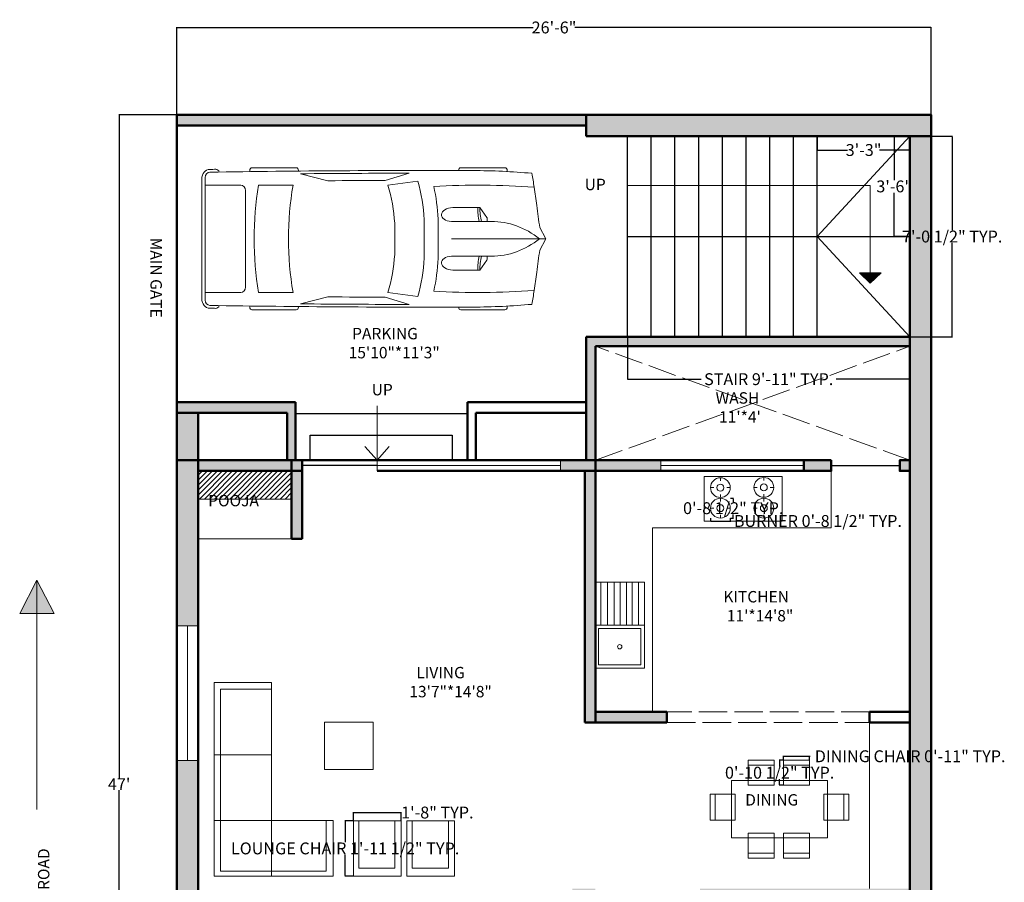
# Model space of a CAD drawing. Units: inches. Extents: x 292 to 1263, y 552 to 1204.
# Tile 2 of 3: x 292 to 707, y 840 to 1204. Entities that reach past the tile are written whole.
import ezdxf

# ---------------------------------------------------------------- set-up
doc = ezdxf.new("R2010")
doc.units = ezdxf.units.IN
doc.header["$MEASUREMENT"] = 0
doc.linetypes.add('ACAD_ISO02W100', pattern=[15, 12, -3])
for name, color, linetype, lineweight in [('A-ANNO-DIMS', 2, 'Continuous', 18), ('A-ANNO-SYMB', 7, 'Continuous', 18), ('A-AREA-IDEN', 30, 'Continuous', 18), ('A-EQPM', 8, 'Continuous', 18), ('A-FLOR-CASE', 92, 'Continuous', 18), ('A-FLOR-CASE-PATT', 252, 'Continuous', 13), ('A-FLOR-FIXT', 9, 'Continuous', 18), ('A-FLOR-OVHD', 8, 'ACAD_ISO02W100', 18), ('A-FLOR-STRS', 7, 'Continuous', 25), ('A-SITE-VEHI', 8, 'Continuous', 18), ('A-WALL-PATT', 22, 'Continuous', 13), ('DOOR', 200, 'Continuous', 25), ('FUR', 92, 'Continuous', 18), ('TEXT', 30, 'Continuous', 18), ('WALL', 22, 'Continuous', 50), ('WIND', 120, 'Continuous', 18)]:
    doc.layers.add(name, color=color, linetype=linetype, lineweight=lineweight)
doc.styles.get("Standard").update_dxf_attribs({"font": 'arial.ttf'})
doc.dimstyles.get("Standard").update_dxf_attribs({"dimtxt": 5, "dimasz": 0.18, "dimexe": 0.18, "dimexo": 0.0625, "dimgap": 0.09, "dimtad": 0, "dimtih": 1, "dimtoh": 1, "dimdec": 0, "dimzin": 0, "dimdsep": 46, "dimlunit": 4, "dimtxsty": 'Standard', "dimcen": 0.09, "dimadec": 0, "dimazin": 0, "dimtfac": 1, "dimtdec": 0, "dimtofl": 0, "dimtmove": 0, "dimatfit": 3, "dimfxl": 1, "dimtolj": 1, "dimtzin": 0, "dimarcsym": 0})

# ---------------------------------------------------------------- blocks, each defined once
blk = doc.blocks.new('*U5')
for p, q in [((46.55, 38.89), (22.35, 38.89)), ((136.7, 38.89), (160.9, 38.89)), ((21.1, 37.41), (21.1, 36.83)), ((47.8, 37.39), (47.8, 37.41)), ((87.99, 31.87), (74.76, 35.92)), ((134.31, 35.6), (119.29, 31.78)), ((135.45, 37.07), (135.45, 37.41)), ((162.15, 37.41), (162.15, 36.77)), ((186.47, -33.5), (186.47, 33.5)), ((188.4, -32.76), (188.4, 32.76)), ((70.03, 31.54), (86.41, 29.35)), ((138.42, 29.35), (157.25, 29.35)), ((186.47, 29.35), (167.01, 29.35)), ((164.52, 26.39), (164.52, -26.39)), ((32.27, 11.63), (36.13, 17.17)), ((36.13, 17.17), (50.94, 17.17)), ((32.12, 9.51), (32.12, 11.15)), ((3.27, 6.13), (0.1, 0.41)), ((29.77, 9.51), (51.68, 9.51)), ((58.92, -10.77), (58.92, 10.77)), ((66.55, -10.53), (66.55, 10.53)), ((82.74, 8.5), (82.74, -8.5)), ((186.47, -10.53), (186.47, 10.53)), ((0, 0), (51.68, 0)), ((0.1, -0.41), (3.27, -6.13)), ((29.77, -9.51), (51.68, -9.51)), ((32.12, -9.51), (32.12, -11.15)), ((32.27, -11.63), (36.13, -17.17)), ((36.13, -17.17), (50.94, -17.17)), ((86.41, -29.35), (70.03, -31.54)), ((87.99, -31.87), (74.76, -35.92)), ((134.31, -35.6), (119.29, -31.78)), ((157.25, -29.35), (138.42, -29.35)), ((167.01, -29.35), (186.47, -29.35)), ((21.1, -37.41), (21.1, -36.83)), ((47.8, -37.39), (47.8, -37.41)), ((135.45, -37.07), (135.45, -37.41)), ((162.15, -37.41), (162.15, -36.77)), ((46.55, -38.89), (22.35, -38.89)), ((136.7, -38.89), (160.9, -38.89))]:
    blk.add_line(p, q)
for centre, major_axis, ratio, start_param, end_param in [((22.35, 37.41), (0, -1.48), 0.842304, 3.141593, 4.712389), ((46.55, 37.41), (0, 1.48), 0.842304, -1.570796, 0), ((136.7, 37.41), (0, -1.48), 0.842304, 3.141593, 4.712389), ((160.9, 37.41), (0, 1.48), 0.842304, -1.570796, 0), ((180.63, 35.84), (0, 2.22), 0.842304, -0.013017, 1.249894), ((64.48, -10556.36), (0, 10595.31), 0.842304, -0.013397, -0.013017), ((183.98, 32.76), (0, -5.25), 0.842304, 1.570796, 3.128196), ((266.03, -27.52), (0, 313.31), 0.842304, 1.367076, 1.39176), ((41.19, -490.86), (0, 528.23), 0.842304, 0.00281, 0.075598), ((64.48, -10555.62), (0, 10593.03), 0.842304, -0.013397, 0.002797), ((64.48, -10555.62), (0, -10591.55), 0.842304, 3.133765, 3.140441), ((183.98, 33.5), (0, -2.96), 0.842304, 1.570796, 3.128196), ((259.18, -27.52), (0, -305.3), 0.842304, 4.528606, 4.561838), ((37.47, -593.96), (0, -623.33), 0.842304, 3.096046, 3.200911), ((134.4, 5.39), (0, -89.78), 0.842304, 4.449482, 4.652344), ((135.29, 5.39), (0, 81.77), 0.842304, 1.245306, 1.50788), ((149.6, 2.8), (0, -79.58), 0.842304, 4.372215, 4.640744), ((95.79, -3666.35), (0, -3698.24), 0.842304, 3.134049, 3.144098), ((17.08, 0), (0, 147.02), 0.842304, 4.511394, 4.913384), ((35.91, 0), (0, 147.02), 0.842304, 4.511394, 4.913384), ((167.01, 26.39), (0, 2.96), 0.842304, 0, 1.570796), ((-204.49, 52.4), (0, -250.96), 0.842304, 1.385369, 1.434372), ((13.04, 17.01), (0, 27.42), 0.842304, 4.435146, 4.718221), ((14.2, 17.01), (0, 27.42), 0.842304, 4.435146, 4.718221), ((50.79, 13.34), (6.34, -0.36), 0.603834, -1.395552, 1.581315), ((32.75, 11.15), (0, 0.74), 0.842304, 0.879714, 1.570796), ((29.77, -46.66), (0, 56.17), 0.842304, 0, 0.590319), ((0.62, 0), (0, -0.74), 0.842304, 4.131459, 5.293319), ((29.77, 46.66), (0, 56.17), 0.842304, 2.551274, 3.141593), ((-204.49, -52.4), (0, 250.96), 0.842304, -1.434372, -1.385369), ((13.04, -17.01), (0, -27.42), 0.842304, 1.564964, 1.848039), ((14.2, -17.01), (0, -27.42), 0.842304, 1.564964, 1.848039), ((134.4, -5.39), (0, -89.78), 0.842304, -1.510751, -1.307889), ((135.29, -5.39), (0, -81.77), 0.842304, -1.50788, -1.245306), ((149.6, -2.8), (0, -79.58), 0.842304, -1.499151, -1.230623), ((32.75, -11.15), (0, -0.74), 0.842304, 4.712389, 5.403472), ((259.18, 27.52), (0, 305.3), 0.842304, 1.721348, 1.754579), ((167.01, -26.39), (0, -2.96), 0.842304, 4.712389, 6.283185), ((266.03, 27.52), (0, 313.31), 0.842304, 1.749832, 1.774517), ((37.47, 593.96), (0, -623.33), 0.842304, -0.059319, 0.045547), ((95.79, 3666.35), (0, -3698.24), 0.842304, -0.002505, 0.007544), ((41.19, 490.86), (0, -528.23), 0.842304, -0.075598, -0.00281), ((22.35, -37.41), (0, 1.48), 0.842304, 1.570796, 3.141593), ((64.48, 10555.62), (0, 10593.03), 0.842304, 3.138796, 3.15499), ((46.55, -37.41), (0, -1.48), 0.842304, 0, 1.570796), ((64.48, 10555.62), (0, -10591.55), 0.842304, 0.001152, 0.007828), ((136.7, -37.41), (0, -1.48), 0.842304, -1.570796, 0), ((160.9, -37.41), (0, 1.48), 0.842304, 3.141593, 4.712389), ((180.63, -35.84), (0, -2.22), 0.842304, -1.249894, 0.013017), ((183.98, -33.5), (0, 2.96), 0.842304, 3.15499, 4.712389), ((183.98, -32.76), (0, -5.25), 0.842304, 0.013397, 1.570796), ((64.48, 10556.36), (0, 10595.31), 0.842304, 3.15461, 3.15499)]:
    blk.add_ellipse(centre, major_axis=major_axis, ratio=ratio, start_param=start_param, end_param=end_param)
at = {"extrusion": (0, 0, -1)}
blk.add_ellipse((50.79, -13.34), major_axis=(6.34, 0.36), ratio=0.603834, start_param=-1.395552, end_param=1.581315, dxfattribs=at)
blk = doc.blocks.new('*D6')
at = {"layer": 'A-ANNO-DIMS', "color": 0, "lineweight": -2, "transparency": 16777216}
for p, q in [((357.97, 1163.71), (357.97, 1200.66)), ((358.15, 1200.48), (508.25, 1200.48)), ((675.79, 1200.48), (525.69, 1200.48)), ((675.97, 1163.71), (675.97, 1200.66))]:
    blk.add_line(p, q, dxfattribs=at)
at = {"layer": 'A-ANNO-DIMS', "color": 0, "lineweight": 100, "transparency": 16777216}
for points in [[(358.15, 1200.51), (358.15, 1200.45), (357.97, 1200.48)], [(675.79, 1200.51), (675.79, 1200.45), (675.97, 1200.48)]]:
    blk.add_solid(points, dxfattribs=at)
at = {"layer": 'Defpoints', "color": 0, "lineweight": 100, "transparency": 16777216}
for p in [(675.97, 1200.48), (357.97, 1163.64), (675.97, 1163.64)]:
    blk.add_point(p, dxfattribs=at)
at = {"layer": 'A-ANNO-DIMS', "color": 0, "transparency": 16777216, "insert": (516.97, 1200.48), "char_height": 5, "attachment_point": 5}
blk.add_mtext('\\A1;26\'-6"', dxfattribs=at)
blk = doc.blocks.new('*D7')
at = {"layer": 'A-ANNO-DIMS', "color": 0, "lineweight": -2, "transparency": 16777216}
for p, q in [((357.91, 1163.64), (333.48, 1163.64)), ((333.66, 1163.46), (333.66, 884.23)), ((333.66, 599.82), (333.66, 879.05)), ((357.91, 599.64), (333.48, 599.64))]:
    blk.add_line(p, q, dxfattribs=at)
at = {"layer": 'A-ANNO-DIMS', "color": 0, "lineweight": 100, "transparency": 16777216}
for points in [[(333.63, 1163.46), (333.69, 1163.46), (333.66, 1163.64)], [(333.63, 599.82), (333.69, 599.82), (333.66, 599.64)]]:
    blk.add_solid(points, dxfattribs=at)
at = {"layer": 'Defpoints', "color": 0, "lineweight": 100, "transparency": 16777216}
for p in [(333.66, 1163.64), (357.97, 1163.64), (357.97, 599.64)]:
    blk.add_point(p, dxfattribs=at)
at = {"layer": 'A-ANNO-DIMS', "color": 0, "transparency": 16777216, "insert": (333.66, 881.64), "char_height": 5, "attachment_point": 5}
blk.add_mtext("\\A1;47'", dxfattribs=at)
blk = doc.blocks.new('*D13')
at = {"layer": 'A-ANNO-DIMS', "color": 0, "lineweight": -2, "transparency": 16777216}
for p, q in [((666.91, 1154.64), (660.2, 1154.64)), ((660.38, 1154.46), (660.38, 1136.16)), ((660.38, 1112.57), (660.38, 1130.87)), ((666.91, 1112.39), (660.2, 1112.39))]:
    blk.add_line(p, q, dxfattribs=at)
at = {"layer": 'A-ANNO-DIMS', "color": 0, "lineweight": 100, "transparency": 16777216}
for points in [[(660.35, 1154.46), (660.41, 1154.46), (660.38, 1154.64)], [(660.35, 1112.57), (660.41, 1112.57), (660.38, 1112.39)]]:
    blk.add_solid(points, dxfattribs=at)
at = {"layer": 'Defpoints', "color": 0, "lineweight": 100, "transparency": 16777216}
for p in [(660.38, 1154.64), (666.97, 1154.64), (666.97, 1112.39)]:
    blk.add_point(p, dxfattribs=at)
at = {"layer": 'A-ANNO-DIMS', "color": 0, "transparency": 16777216, "insert": (660.38, 1133.52), "char_height": 5, "attachment_point": 5}
blk.add_mtext('\\A1;3\'-6"', dxfattribs=at)
blk = doc.blocks.new('*D14')
at = {"layer": 'A-ANNO-DIMS', "color": 0, "lineweight": -2, "transparency": 16777216}
for p, q in [((627.97, 1154.58), (627.97, 1148.67)), ((666.97, 1154.58), (666.97, 1148.67)), ((628.15, 1148.85), (640.73, 1148.85)), ((666.79, 1148.85), (654.2, 1148.85))]:
    blk.add_line(p, q, dxfattribs=at)
at = {"layer": 'A-ANNO-DIMS', "color": 0, "lineweight": 100, "transparency": 16777216}
for points in [[(628.15, 1148.88), (628.15, 1148.82), (627.97, 1148.85)], [(666.79, 1148.88), (666.79, 1148.82), (666.97, 1148.85)]]:
    blk.add_solid(points, dxfattribs=at)
at = {"layer": 'Defpoints', "color": 0, "lineweight": 100, "transparency": 16777216}
for p in [(627.97, 1154.64), (666.97, 1154.64), (666.97, 1148.85)]:
    blk.add_point(p, dxfattribs=at)
at = {"layer": 'A-ANNO-DIMS', "color": 0, "transparency": 16777216, "insert": (647.47, 1148.85), "char_height": 5, "attachment_point": 5}
blk.add_mtext('\\A1;3\'-3"', dxfattribs=at)
blk = doc.blocks.new('SOFA-SECTIONAL')
for p, q in [((2.73, 2.04), (2.73, 78.73)), ((2.73, 78.73), (24.15, 78.73)), ((24.15, 51.12), (0, 51.12)), ((47.26, 23.35), (47.26, 2.04)), ((47.26, 2.04), (2.73, 2.04))]:
    blk.add_line(p, q)
for points in [[(0, 0), (24.15, 0), (24.15, 81.48), (0, 81.48)], [(0, 0), (50.13, 0), (50.13, 23.35), (0, 23.35)]]:
    blk.add_lwpolyline(points, close=True)
blk = doc.blocks.new('CHAIR-LOUNGE')
for p, q in [((2.25, 23.26), (2.25, 3.36)), ((17.47, 3.36), (17.47, 23.26)), ((2.25, 3.36), (17.47, 3.36))]:
    blk.add_line(p, q)
blk.add_lwpolyline([(0, 0), (20.12, 0), (20.12, 23.26), (0, 23.26)], close=True)
blk = doc.blocks.new('CHAIR-DINING')
blk.add_line((0, 8.43), (11, 8.43))
blk.add_lwpolyline([(0, 0), (11, 0), (11, 10.56), (0, 10.56)], close=True)
blk = doc.blocks.new('COOKTOP-BURNER')
for p, q in [((4.16, 8.32), (4.16, 7.02)), ((0, 4.16), (0.93, 4.16)), ((0, 4.16), (1.41, 4.16)), ((6.9, 4.16), (8.32, 4.16)), ((4.16, 1.29), (4.16, 0))]:
    blk.add_line(p, q)
for radius in [4.16, 1.47]:
    blk.add_circle((4.16, 4.16), radius)
blk = doc.blocks.new('STAIR-RETURN')
for p, q in [((0, 0), (0, 84.5)), ((10, 0), (10, 84.5)), ((20, 0), (20, 84.5)), ((30, 0), (30, 84.5)), ((40, 0), (40, 84.5)), ((50, 0), (50, 84.5)), ((60, 0), (60, 84.5)), ((70, 0), (70, 84.5)), ((80, 0), (80, 84.5)), ((80, 42.25), (119, 84.5)), ((0, 42.25), (119, 42.25)), ((80, 42.25), (119, 0)), ((80, 0), (80, 39))]:
    blk.add_line(p, q)
blk = doc.blocks.new('STAIR-TRAVEL-ARROW')
h = blk.add_hatch()
h.set_pattern_fill('ANSI31', color=256)
h.set_pattern_definition([(45, (-547.968, -1092.695), (-0.088388348, 0.088388348), [])])
h.paths.add_polyline_path([(102.33, 4.46), (97.71, 4.46), (102.33, 0)])
h.paths.add_polyline_path([(106.95, 4.46), (102.33, 4.46), (102.33, 0)])
for p, q in [((0, 41.14), (102.33, 41.14)), ((102.33, 41.14), (102.33, 0)), ((102.33, 0), (97.71, 4.46)), ((97.71, 4.46), (106.95, 4.46)), ((102.33, 0), (106.95, 4.46))]:
    blk.add_line(p, q)
blk = doc.blocks.new('ROAD-DIRECTION')
h = blk.add_hatch(color=256)
h.dxf.hatch_style = 1
h.paths.add_polyline_path([(7.26, 265.02), (0, 250.97), (7.26, 250.97)])
h.paths.add_polyline_path([(7.26, 265.02), (7.26, 250.97), (14.53, 250.97)])
h.paths.add_polyline_path([(14.53, 14.04), (7.26, 14.04), (7.26, 0)])
h.paths.add_polyline_path([(7.26, 14.04), (0, 14.04), (7.26, 0)])
for p, q in [((7.26, 265.02), (0, 250.97)), ((7.26, 168.49), (7.26, 265.02)), ((7.26, 265.02), (14.53, 250.97)), ((0, 250.97), (14.53, 250.97)), ((7.26, 96.52), (7.26, 0)), ((7.26, 0), (0, 14.04)), ((0, 14.04), (14.53, 14.04)), ((7.26, 0), (14.53, 14.04))]:
    blk.add_line(p, q)
blk = doc.blocks.new('WASH-VOID')
for p, q in [((0, 0), (132.5, 48)), ((132.5, 0), (0, 48))]:
    blk.add_line(p, q)
blk = doc.blocks.new('WIN-SIDE')
blk.add_line((4.5, 0), (4.5, 56.83))
blk.add_lwpolyline([(9, 56.83), (0, 56.83), (0, 0), (9, 0)], close=True)
blk = doc.blocks.new('*D29')
at = {"layer": 'A-ANNO-DIMS', "color": 0, "lineweight": -2, "transparency": 16777216}
for p, q in [((613.73, 891.82), (613.73, 893.58)), ((613.91, 893.4), (624.55, 893.4)), ((624.73, 891.82), (624.73, 893.58)), ((624.73, 893.4), (624.91, 893.4))]:
    blk.add_line(p, q, dxfattribs=at)
at = {"layer": 'A-ANNO-DIMS', "color": 0, "lineweight": 100, "transparency": 16777216}
for points in [[(613.91, 893.43), (613.91, 893.37), (613.73, 893.4)], [(624.55, 893.43), (624.55, 893.37), (624.73, 893.4)]]:
    blk.add_solid(points, dxfattribs=at)
at = {"layer": 'Defpoints', "color": 0, "lineweight": 100, "transparency": 16777216}
for p in [(624.73, 893.4), (613.73, 891.75), (624.73, 891.75)]:
    blk.add_point(p, dxfattribs=at)
at = {"layer": 'A-ANNO-DIMS', "color": 0, "transparency": 16777216, "insert": (667.09, 893.4), "char_height": 5, "attachment_point": 5}
blk.add_mtext('\\A1;DINING CHAIR 0\'-11" TYP.', dxfattribs=at)
blk = doc.blocks.new('*D30')
at = {"layer": 'A-ANNO-DIMS', "color": 0, "lineweight": -2, "transparency": 16777216}
for p, q in [((613.67, 891.75), (611.9, 891.75)), ((612.08, 891.57), (612.08, 889.15)), ((613.67, 881.19), (611.9, 881.19)), ((612.08, 881.37), (612.08, 883.8))]:
    blk.add_line(p, q, dxfattribs=at)
at = {"layer": 'A-ANNO-DIMS', "color": 0, "lineweight": 100, "transparency": 16777216}
for points in [[(612.05, 891.57), (612.11, 891.57), (612.08, 891.75)], [(612.05, 881.37), (612.11, 881.37), (612.08, 881.19)]]:
    blk.add_solid(points, dxfattribs=at)
at = {"layer": 'Defpoints', "color": 0, "lineweight": 100, "transparency": 16777216}
for p in [(612.08, 891.75), (613.73, 891.75), (613.73, 881.19)]:
    blk.add_point(p, dxfattribs=at)
at = {"layer": 'A-ANNO-DIMS', "color": 0, "transparency": 16777216, "insert": (612.08, 886.47), "char_height": 5, "attachment_point": 5}
blk.add_mtext('\\A1;0\'-10 1/2" TYP.', dxfattribs=at)
blk = doc.blocks.new('*D31')
at = {"layer": 'A-ANNO-DIMS', "color": 0, "lineweight": -2, "transparency": 16777216}
for p, q in [((582.96, 993.71), (582.96, 992.35)), ((583.14, 992.53), (591.09, 992.53)), ((591.27, 993.71), (591.27, 992.35)), ((591.27, 992.53), (591.45, 992.53))]:
    blk.add_line(p, q, dxfattribs=at)
at = {"layer": 'A-ANNO-DIMS', "color": 0, "lineweight": 100, "transparency": 16777216}
for points in [[(583.14, 992.56), (583.14, 992.5), (582.96, 992.53)], [(591.09, 992.56), (591.09, 992.5), (591.27, 992.53)]]:
    blk.add_solid(points, dxfattribs=at)
at = {"layer": 'Defpoints', "color": 0, "lineweight": 100, "transparency": 16777216}
for p in [(582.96, 993.78), (591.27, 993.78), (591.27, 992.53)]:
    blk.add_point(p, dxfattribs=at)
at = {"layer": 'A-ANNO-DIMS', "color": 0, "transparency": 16777216, "insert": (628.21, 992.53), "char_height": 5, "attachment_point": 5}
blk.add_mtext('\\A1;BURNER 0\'-8 1/2" TYP.', dxfattribs=at)
blk = doc.blocks.new('*D32')
at = {"layer": 'A-ANNO-DIMS', "color": 0, "lineweight": -2, "transparency": 16777216}
for p, q in [((591.33, 1002.09), (592.7, 1002.09)), ((592.52, 1001.91), (592.52, 1000.61)), ((591.33, 993.78), (592.7, 993.78)), ((592.52, 993.96), (592.52, 995.26))]:
    blk.add_line(p, q, dxfattribs=at)
at = {"layer": 'A-ANNO-DIMS', "color": 0, "lineweight": 100, "transparency": 16777216}
for points in [[(592.49, 1001.91), (592.55, 1001.91), (592.52, 1002.09)], [(592.49, 993.96), (592.55, 993.96), (592.52, 993.78)]]:
    blk.add_solid(points, dxfattribs=at)
at = {"layer": 'Defpoints', "color": 0, "lineweight": 100, "transparency": 16777216}
for p in [(591.27, 1002.09), (592.52, 1002.09), (591.27, 993.78)]:
    blk.add_point(p, dxfattribs=at)
at = {"layer": 'A-ANNO-DIMS', "color": 0, "transparency": 16777216, "insert": (592.52, 997.94), "char_height": 5, "attachment_point": 5}
blk.add_mtext('\\A1;0\'-8 1/2" TYP.', dxfattribs=at)
blk = doc.blocks.new('*D37')
at = {"layer": 'A-ANNO-DIMS', "color": 0, "lineweight": -2, "transparency": 16777216}
for p, q in [((432.33, 866.2), (428.73, 866.2)), ((428.91, 866.02), (428.91, 857.25)), ((428.91, 843.12), (428.91, 851.9)), ((432.33, 842.94), (428.73, 842.94))]:
    blk.add_line(p, q, dxfattribs=at)
at = {"layer": 'A-ANNO-DIMS', "color": 0, "lineweight": 100, "transparency": 16777216}
for points in [[(428.88, 866.02), (428.94, 866.02), (428.91, 866.2)], [(428.88, 843.12), (428.94, 843.12), (428.91, 842.94)]]:
    blk.add_solid(points, dxfattribs=at)
at = {"layer": 'Defpoints', "color": 0, "lineweight": 100, "transparency": 16777216}
for p in [(428.91, 866.2), (432.4, 866.2), (432.4, 842.94)]:
    blk.add_point(p, dxfattribs=at)
at = {"layer": 'A-ANNO-DIMS', "color": 0, "transparency": 16777216, "insert": (428.91, 854.57), "char_height": 5, "attachment_point": 5}
blk.add_mtext('\\A1;LOUNGE CHAIR 1\'-11 1/2" TYP.', dxfattribs=at)
blk = doc.blocks.new('*D38')
at = {"layer": 'A-ANNO-DIMS', "color": 0, "lineweight": -2, "transparency": 16777216}
for p, q in [((432.4, 866.27), (432.4, 869.87)), ((432.58, 869.69), (452.33, 869.69)), ((452.51, 866.27), (452.51, 869.87)), ((452.51, 869.69), (452.69, 869.69))]:
    blk.add_line(p, q, dxfattribs=at)
at = {"layer": 'A-ANNO-DIMS', "color": 0, "lineweight": 100, "transparency": 16777216}
for points in [[(432.58, 869.72), (432.58, 869.66), (432.4, 869.69)], [(452.33, 869.72), (452.33, 869.66), (452.51, 869.69)]]:
    blk.add_solid(points, dxfattribs=at)
at = {"layer": 'Defpoints', "color": 0, "lineweight": 100, "transparency": 16777216}
for p in [(452.51, 869.69), (432.4, 866.2), (452.51, 866.2)]:
    blk.add_point(p, dxfattribs=at)
at = {"layer": 'A-ANNO-DIMS', "color": 0, "transparency": 16777216, "insert": (467.79, 869.69), "char_height": 5, "attachment_point": 5}
blk.add_mtext('\\A1;1\'-8" TYP.', dxfattribs=at)
blk = doc.blocks.new('*D39')
at = {"layer": 'A-ANNO-DIMS', "color": 0, "lineweight": -2, "transparency": 16777216}
for p, q in [((547.97, 1070.08), (547.97, 1052.11)), ((666.97, 1070.08), (666.97, 1052.11)), ((548.15, 1052.29), (578.95, 1052.29)), ((666.79, 1052.29), (635.98, 1052.29))]:
    blk.add_line(p, q, dxfattribs=at)
at = {"layer": 'A-ANNO-DIMS', "color": 0, "lineweight": 100, "transparency": 16777216}
for points in [[(548.15, 1052.32), (548.15, 1052.26), (547.97, 1052.29)], [(666.79, 1052.32), (666.79, 1052.26), (666.97, 1052.29)]]:
    blk.add_solid(points, dxfattribs=at)
at = {"layer": 'Defpoints', "color": 0, "lineweight": 100, "transparency": 16777216}
for p in [(547.97, 1070.14), (666.97, 1070.14), (666.97, 1052.29)]:
    blk.add_point(p, dxfattribs=at)
at = {"layer": 'A-ANNO-DIMS', "color": 0, "transparency": 16777216, "insert": (607.47, 1052.29), "char_height": 5, "attachment_point": 5}
blk.add_mtext('\\A1;STAIR 9\'-11" TYP.', dxfattribs=at)
blk = doc.blocks.new('*D40')
at = {"layer": 'A-ANNO-DIMS', "color": 0, "lineweight": -2, "transparency": 16777216}
for p, q in [((667.03, 1154.64), (685, 1154.64)), ((684.82, 1154.46), (684.82, 1115.07)), ((684.82, 1070.32), (684.82, 1109.72)), ((667.03, 1070.14), (685, 1070.14))]:
    blk.add_line(p, q, dxfattribs=at)
at = {"layer": 'A-ANNO-DIMS', "color": 0, "lineweight": 100, "transparency": 16777216}
for points in [[(684.79, 1154.46), (684.85, 1154.46), (684.82, 1154.64)], [(684.79, 1070.32), (684.85, 1070.32), (684.82, 1070.14)]]:
    blk.add_solid(points, dxfattribs=at)
at = {"layer": 'Defpoints', "color": 0, "lineweight": 100, "transparency": 16777216}
for p in [(666.97, 1154.64), (684.82, 1154.64), (666.97, 1070.14)]:
    blk.add_point(p, dxfattribs=at)
at = {"layer": 'A-ANNO-DIMS', "color": 0, "transparency": 16777216, "insert": (684.82, 1112.39), "char_height": 5, "attachment_point": 5}
blk.add_mtext('\\A1;7\'-0 1/2" TYP.', dxfattribs=at)

msp = doc.modelspace()

# ---------------------------------------------------------------- hatches: boundary and pattern name
at = {"layer": 'A-FLOR-CASE-PATT'}
h = msp.add_hatch(dxfattribs=at)
h.set_pattern_fill('ANSI31', color=256, scale=12)
h.paths.add_polyline_path([(406.28, 1013.64), (366.97, 1013.64), (366.97, 1001.8), (406.28, 1001.8)])
at = {"layer": 'A-WALL-PATT'}
h = msp.add_hatch(color=256, dxfattribs=at)
h.dxf.hatch_style = 1
h.paths.add_polyline_path([(530.47, 1163.64), (357.97, 1163.64), (357.97, 1159.14), (530.47, 1159.14)])
h.paths.add_polyline_path([(407.97, 1042.64), (357.97, 1042.64), (357.97, 1038.14), (404.42, 1038.14), (404.42, 1018.14), (407.97, 1018.14)])
h = msp.add_hatch(color=256, dxfattribs=at)
h.dxf.hatch_style = 1
h.paths.add_polyline_path([(675.97, 1163.64), (530.47, 1163.64), (530.47, 1154.64), (675.97, 1154.64)])
h = msp.add_hatch(color=256, dxfattribs=at)
h.dxf.hatch_style = 1
h.paths.add_polyline_path([(675.97, 1154.64), (666.97, 1154.64), (666.97, 599.64), (675.97, 599.64)])
h.paths.add_polyline_path([(666.97, 608.64), (644.63, 608.64), (644.63, 599.64), (666.97, 599.64)])
h.paths.add_polyline_path([(469.97, 713.14), (406.46, 713.14), (406.46, 708.64), (469.97, 708.64)])
h = msp.add_hatch(color=256, dxfattribs=at)
h.dxf.hatch_style = 1
h.paths.add_polyline_path([(534.47, 1013.64), (529.97, 1013.64), (529.97, 907.64), (534.47, 907.64)])
h.paths.add_polyline_path([(666.97, 1070.14), (627.97, 1070.14), (530.47, 1070.14), (530.47, 1018.14), (534.47, 1018.14), (534.47, 1066.14), (666.97, 1066.14)])
h.paths.add_polyline_path([(633.82, 1018.14), (622.22, 1018.14), (622.22, 1013.64), (633.82, 1013.64)])
h.paths.add_polyline_path([(562.03, 1018.14), (534.97, 1018.14), (534.47, 1018.14), (534.47, 1013.64), (562.03, 1013.64)])
h.paths.add_polyline_path([(666.97, 1018.14), (662.7, 1018.14), (662.7, 1013.64), (666.97, 1013.64)])
h.paths.add_polyline_path([(534.47, 1018.14), (519.71, 1018.14), (519.71, 1013.64), (529.97, 1013.64), (534.47, 1013.64)])
h = msp.add_hatch(color=256, dxfattribs=at)
h.dxf.hatch_style = 1
h.paths.add_polyline_path([(366.97, 1038.14), (357.97, 1038.14), (357.97, 1018.14), (366.97, 1018.14)])
h.paths.add_polyline_path([(366.97, 1013.64), (366.97, 1018.14), (357.97, 1018.14), (357.97, 948.4), (366.97, 948.4)])
h.paths.add_polyline_path([(366.97, 891.57), (357.97, 891.57), (357.97, 803.1), (366.97, 803.1), (366.97, 833.14)])
h.paths.add_polyline_path([(366.97, 746.27), (357.97, 746.27), (357.97, 702.82), (366.97, 702.82), (366.97, 708.64)])
h.paths.add_polyline_path([(381.13, 608.64), (367.97, 608.64), (366.97, 608.64), (366.97, 618.29), (357.97, 618.29), (357.97, 599.64), (381.13, 599.64)])
h.paths.add_polyline_path([(492.73, 608.64), (474.47, 608.64), (469.6, 608.64), (469.6, 599.64), (492.73, 599.64)])
h.paths.add_polyline_path([(560.01, 608.64), (516.97, 608.64), (516.97, 599.64), (560.01, 599.64)])
h.paths.add_polyline_path([(474.47, 708.64), (474.47, 713.14), (469.97, 713.14), (469.97, 608.64), (474.47, 608.64)])
h.paths.add_polyline_path([(534.97, 764.64), (534.92, 775.88), (534.43, 837.64), (524.76, 837.64), (524.76, 833.14), (529.97, 833.14), (530.47, 769.14), (530.47, 608.64), (534.97, 608.64)])
h.paths.add_polyline_path([(582.97, 769.14), (582.97, 775.01), (578.47, 775.01), (578.47, 769.14), (578.47, 739.47), (582.97, 739.47), (582.97, 764.64)])
h.paths.add_polyline_path([(666.97, 769.14), (642.97, 769.14), (582.97, 769.14), (582.97, 764.64), (666.97, 764.64)])
h.paths.add_polyline_path([(666.97, 837.64), (578.47, 837.64), (578.47, 816.16), (578.47, 815.01), (582.97, 815.01), (582.97, 816.16), (582.97, 833.14), (666.97, 833.14)])
h.paths.add_polyline_path([(564.59, 912.14), (534.47, 912.14), (534.47, 907.64), (564.59, 907.64)])
h = msp.add_hatch(color=256, dxfattribs=at)
h.dxf.hatch_style = 1
h.paths.add_polyline_path([(410.78, 1013.64), (406.28, 1013.64), (406.28, 984.99), (410.78, 984.99)])
h.paths.add_polyline_path([(410.78, 1018.14), (406.28, 1018.14), (406.28, 1013.64), (410.78, 1013.64)])
h.paths.add_polyline_path([(406.28, 1018.14), (366.97, 1018.14), (366.97, 1013.64), (406.28, 1013.64)])

# ---------------------------------------------------------------- linework, layer by layer
at = {"layer": 'A-ANNO-SYMB'}
for p, q in [((442.36, 1037.79), (442.36, 1041.1)), ((442.36, 1018.14), (442.36, 1037.79)), ((442.36, 1018.14), (437.25, 1023.93)), ((442.36, 1018.14), (447.46, 1023.93))]:
    msp.add_line(p, q, dxfattribs=at)
at = {"layer": 'A-EQPM'}
msp.add_lwpolyline([(580.24, 1011.26), (613.12, 1011.26), (613.12, 992.46), (580.24, 992.46)], close=True, dxfattribs=at)
at = {"layer": 'A-FLOR-CASE'}
for p, q in [((633.82, 1013.64), (633.82, 989.64)), ((366.97, 1001.8), (406.28, 1001.8)), ((633.82, 989.64), (558.47, 989.64)), ((558.47, 912.14), (558.47, 989.64)), ((406.28, 984.99), (366.97, 984.99)), ((534.47, 912.14), (558.47, 912.14)), ((650.02, 907.64), (650.02, 837.64))]:
    msp.add_line(p, q, dxfattribs=at)
at = {"layer": 'A-FLOR-FIXT'}
for p, q in [((536.76, 948.66), (536.76, 966.8)), ((539.45, 948.66), (539.45, 966.8)), ((542.32, 948.66), (542.32, 966.8)), ((544.92, 948.66), (544.92, 966.8)), ((547.52, 948.67), (547.52, 966.81)), ((549.94, 948.67), (549.94, 966.81)), ((552.54, 948.66), (552.54, 966.8)), ((555.11, 948.66), (534.47, 948.66))]:
    msp.add_line(p, q, dxfattribs=at)
for points in [[(555.11, 966.8), (534.47, 966.8), (534.47, 930.52), (555.11, 930.52)], [(535.78, 931.94), (553.61, 931.94), (553.61, 947.17), (535.78, 947.17)]]:
    msp.add_lwpolyline(points, close=True, dxfattribs=at)
msp.add_circle((544.69, 939.56), 0.924, dxfattribs=at)
at = {"layer": 'A-FLOR-OVHD'}
msp.add_lwpolyline([(564.59, 907.64), (650.02, 907.64), (650.02, 912.14), (564.59, 912.14)], close=True, dxfattribs=at)
at = {"layer": 'A-FLOR-STRS'}
for p, q in [((666.97, 1070.14), (627.97, 1070.14)), ((666.97, 1070.14), (627.97, 1070.14)), ((407.97, 1037.79), (480.47, 1037.79)), ((414.2, 1018.14), (414.2, 1028.7)), ((414.2, 1028.7), (473.97, 1028.7)), ((473.97, 1028.7), (473.97, 1018.14))]:
    msp.add_line(p, q, dxfattribs=at)
at = {"layer": 'DOOR'}
for p, q in [((442.36, 1015.89), (410.78, 1015.89)), ((633.82, 1015.89), (662.7, 1015.89))]:
    msp.add_line(p, q, dxfattribs=at)
at = {"layer": 'FUR'}
for points in [[(420.2, 907.83), (440.72, 907.83), (440.72, 887.85), (420.2, 887.85)], [(591.83, 883.13), (632.25, 883.13), (632.25, 859.07), (591.83, 859.07)]]:
    msp.add_lwpolyline(points, close=True, dxfattribs=at)
at = {"layer": 'WALL'}
for p, q in [((357.97, 1163.64), (675.97, 1163.64)), ((357.97, 1163.64), (357.97, 1159.14)), ((357.97, 1018.14), (357.97, 1163.64)), ((530.47, 1154.64), (530.47, 1163.64)), ((675.97, 599.64), (675.97, 1163.64)), ((530.47, 1159.14), (357.97, 1159.14)), ((530.47, 1154.64), (666.97, 1154.64)), ((666.97, 608.64), (666.97, 1154.64)), ((530.47, 1018.14), (530.47, 1070.14)), ((530.47, 1070.14), (666.97, 1070.14)), ((534.47, 1018.14), (534.47, 1066.14)), ((534.47, 1066.14), (666.97, 1066.14)), ((357.97, 1042.64), (407.97, 1042.64)), ((407.97, 1042.64), (407.97, 1018.14)), ((530.47, 1042.64), (480.47, 1042.64)), ((480.47, 1042.64), (480.47, 1018.14)), ((357.97, 1018.14), (357.97, 1038.14)), ((357.97, 1038.14), (404.42, 1038.14)), ((366.97, 1018.14), (366.97, 1038.14)), ((404.42, 1018.14), (404.42, 1038.14)), ((530.47, 1038.14), (484.01, 1038.14)), ((484.01, 1018.14), (484.01, 1038.14)), ((366.97, 1018.14), (357.97, 1018.14)), ((357.97, 1018.14), (357.97, 599.64)), ((366.97, 1018.14), (366.97, 608.64)), ((366.97, 1018.14), (534.47, 1018.14)), ((406.28, 1018.14), (406.28, 984.99)), ((410.78, 1018.14), (410.78, 984.99)), ((529.97, 1018.14), (633.82, 1018.14)), ((534.47, 1018.14), (534.47, 907.64)), ((633.82, 1018.14), (534.97, 1018.14)), ((666.97, 1018.14), (662.7, 1018.14)), ((662.7, 1018.14), (666.97, 1018.14)), ((366.97, 837.64), (366.97, 1013.64)), ((366.97, 1013.64), (410.78, 1013.64)), ((442.36, 1013.64), (529.97, 1013.64)), ((529.97, 1013.64), (529.97, 907.64)), ((529.97, 1013.64), (633.82, 1013.64)), ((534.47, 1013.64), (534.47, 907.64)), ((662.7, 1013.64), (666.97, 1013.64)), ((406.28, 984.99), (410.78, 984.99)), ((564.59, 912.14), (534.47, 912.14)), ((666.97, 912.14), (650.02, 912.14)), ((534.47, 907.64), (529.97, 907.64)), ((564.59, 907.64), (534.47, 907.64)), ((666.97, 907.64), (650.02, 907.64))]:
    msp.add_line(p, q, dxfattribs=at)
for points in [[(530.47, 1154.64), (675.97, 1154.64), (675.97, 1163.64), (530.47, 1163.64)], [(666.97, 1154.64), (675.97, 1154.64), (675.97, 599.64), (666.97, 599.64)], [(633.82, 1018.14), (622.22, 1018.14), (622.22, 1013.64), (633.82, 1013.64)], [(666.97, 1018.14), (662.7, 1018.14), (662.7, 1013.64), (666.97, 1013.64)]]:
    msp.add_lwpolyline(points, close=True, dxfattribs=at)
for points in [[(564.59, 912.14), (564.59, 907.64)], [(650.02, 907.64), (650.02, 912.14)]]:
    msp.add_lwpolyline(points, dxfattribs=at)
at = {"layer": 'WIND'}
for p, q in [((442.36, 1015.89), (519.71, 1015.89)), ((562.03, 1015.89), (622.22, 1015.89))]:
    msp.add_line(p, q, dxfattribs=at)
for points in [[(519.71, 1013.64), (442.36, 1013.64), (442.36, 1018.14), (519.71, 1018.14)], [(622.22, 1013.64), (562.03, 1013.64), (562.03, 1018.14), (622.22, 1018.14)]]:
    msp.add_lwpolyline(points, close=True, dxfattribs=at)
msp.add_lwpolyline([(473.94, 1013.64), (519.71, 1013.64), (519.71, 1018.14), (473.94, 1018.14)], dxfattribs=at)

# ---------------------------------------------------------------- block references
at = {"layer": 'A-ANNO-SYMB'}
for name, p in [('STAIR-TRAVEL-ARROW', (547.97, 1092.69)), ('ROAD-DIRECTION', (291.73, 702.52))]:
    msp.add_blockref(name, p, dxfattribs=at)
at = {"layer": 'A-EQPM'}
for p in [(582.96, 1002.42), (601.26, 1002.54), (582.96, 993.78), (601.26, 993.78)]:
    msp.add_blockref('COOKTOP-BURNER', p, dxfattribs=at)
at = {"layer": 'A-FLOR-OVHD'}
msp.add_blockref('WASH-VOID', (534.47, 1018.14), dxfattribs=at)
at = {"layer": 'A-FLOR-STRS'}
msp.add_blockref('STAIR-RETURN', (547.97, 1070.14), dxfattribs=at)
at = {"layer": 'A-SITE-VEHI', "xscale": -0.7697678212056502, "yscale": 0.7697678212056502, "zscale": 0.7697678212056502}
msp.add_blockref('*U5', (513.5, 1111.43), dxfattribs=at)
at = {"layer": 'FUR'}
for name, p in [('SOFA-SECTIONAL', (373.7, 842.94)), ('CHAIR-DINING', (598.8, 881.19)), ('CHAIR-DINING', (613.73, 881.19)), ('CHAIR-LOUNGE', (432.4, 842.94)), ('CHAIR-LOUNGE', (454.97, 842.94))]:
    msp.add_blockref(name, p, dxfattribs=at)
at = {"layer": 'FUR', "rotation": 90}
msp.add_blockref('CHAIR-DINING', (593.33, 866.49), dxfattribs=at)
at = {"layer": 'FUR', "extrusion": (0, 0, -1), "zscale": -1}
for p, rotation in [((-630.75, 866.49), 90.0000000000006), ((-598.8, 861.01), 180), ((-613.73, 861.01), 180)]:
    msp.add_blockref('CHAIR-DINING', p, dxfattribs=dict(at, rotation=rotation))
at = {"layer": 'WIND'}
msp.add_blockref('WIN-SIDE', (357.97, 891.57), dxfattribs=at)

# ---------------------------------------------------------------- texts
at = {"layer": 'A-AREA-IDEN', "attachment_point": 1}
for s, insert, char_height in [(' PARKING \\P15\'10"*11\'3"', (430.41, 1073.89), 4.8055), ("WASH\\P 11'*4'", (585.08, 1046.78), 4.805), ('POOJA', (371.2, 1003.52), 4.805), ('KITCHEN\\P 11\'*14\'8"', (588.37, 963.03), 4.805), ('  LIVING\\P13\'7"*14\'8"', (455.99, 931.05), 4.8055), ('DINING', (597.58, 877.43), 4.805)]:
    msp.add_mtext_dynamic_manual_height_columns(s, width=2330.1292, gutter_width=24.03, heights=[0], dxfattribs=dict(at, insert=insert, char_height=char_height))
at = {"layer": 'TEXT', "char_height": 4.805, "attachment_point": 1}
for insert in [(529.9, 1136.74), (440.12, 1050.28)]:
    msp.add_mtext_dynamic_manual_height_columns('UP', width=2330.1292, gutter_width=24.03, heights=[0], dxfattribs=dict(at, insert=insert))
for s, insert, rotation in [('MAIN GATE', (351.66, 1111.9), 270), ('MAIN ROAD', (299.44, 819.63), 90)]:
    msp.add_mtext_dynamic_manual_height_columns(s, width=2330.1292, gutter_width=24.03, heights=[0], dxfattribs=dict(at, insert=insert, rotation=rotation))

# ---------------------------------------------------------------- dimensions: what is measured, and where the dimension line sits
at = {"layer": 'A-ANNO-DIMS'}
for base, p1, p2, picture, middle in [((675.97, 1200.48), (357.97, 1163.64), (675.97, 1163.64), '*D6', (516.97, 1200.48)), ((666.97, 1148.85), (627.97, 1154.64), (666.97, 1154.64), '*D14', (647.47, 1148.85))]:
    dim = msp.add_linear_dim(base=base, p1=p1, p2=p2, dimstyle='Standard', override={"dimclrd": 0, "dimclre": 0, "dimclrt": 0}, dxfattribs=at)
    dim.commit()
    dim.dimension.update_dxf_attribs({"geometry": picture, "text_midpoint": middle})
for base, p1, p2, picture, middle in [((333.66, 1163.64), (357.97, 599.64), (357.97, 1163.64), '*D7', (333.66, 881.64)), ((660.38, 1154.64), (666.97, 1112.39), (666.97, 1154.64), '*D13', (660.38, 1133.52))]:
    dim = msp.add_linear_dim(base=base, p1=p1, p2=p2, angle=90, dimstyle='Standard', override={"dimclrd": 0, "dimclre": 0, "dimclrt": 0}, dxfattribs=at)
    dim.commit()
    dim.dimension.update_dxf_attribs({"geometry": picture, "text_midpoint": middle})
for base, p1, p2, text, picture, middle in [((684.82, 1154.64), (666.97, 1070.14), (666.97, 1154.64), '<> TYP.', '*D40', (684.82, 1112.39)), ((592.52, 1002.09), (591.27, 993.78), (591.27, 1002.09), '<> TYP.', '*D32', (592.52, 997.94)), ((612.08, 891.75), (613.73, 881.19), (613.73, 891.75), '<> TYP.', '*D30', (612.08, 886.47)), ((428.91, 866.2), (432.4, 842.94), (432.4, 866.2), 'LOUNGE CHAIR <> TYP.', '*D37', (428.91, 854.57))]:
    dim = msp.add_linear_dim(base=base, p1=p1, p2=p2, angle=90, text=text, dimstyle='Standard', override={"dimdec": 1, "dimlfac": 1, "dimrnd": 0, "dimzin": 1, "dimdsep": 46, "dimlunit": 4, "dimfrac": 2}, dxfattribs=at)
    dim.commit()
    dim.dimension.update_dxf_attribs({"geometry": picture, "text_midpoint": middle})
for base, p1, p2, text, picture, middle in [((666.97, 1052.29), (547.97, 1070.14), (666.97, 1070.14), 'STAIR <> TYP.', '*D39', (607.47, 1052.29)), ((591.27, 992.53), (582.96, 993.78), (591.27, 993.78), 'BURNER <> TYP.', '*D31', (628.21, 992.53)), ((624.73, 893.4), (613.73, 891.75), (624.73, 891.75), 'DINING CHAIR <> TYP.', '*D29', (667.09, 893.4)), ((452.51, 869.69), (432.4, 866.2), (452.51, 866.2), '<> TYP.', '*D38', (467.79, 869.69))]:
    dim = msp.add_linear_dim(base=base, p1=p1, p2=p2, text=text, dimstyle='Standard', override={"dimdec": 1, "dimlfac": 1, "dimrnd": 0, "dimzin": 1, "dimdsep": 46, "dimlunit": 4, "dimfrac": 2}, dxfattribs=at)
    dim.commit()
    dim.dimension.update_dxf_attribs({"geometry": picture, "text_midpoint": middle})

doc.saveas('drawing.dxf')
